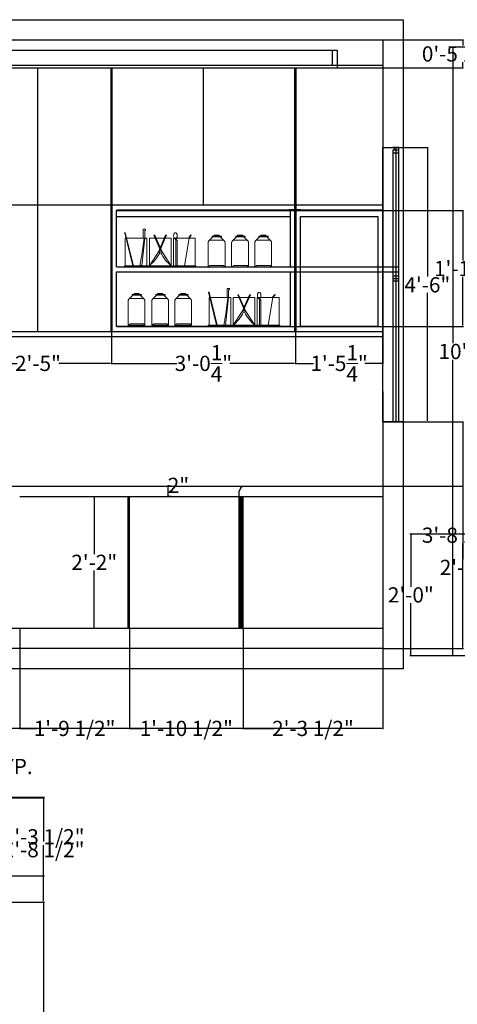
# Model space of a CAD drawing. Units: inches. Extents: x 1686244 to 1686928, y 1936095 to 1936489.
# Tile 9 of 11: x 1686616 to 1686702, y 1936281 to 1936475. Entities that reach past the tile are written whole.
import ezdxf

# ---------------------------------------------------------------- set-up
doc = ezdxf.new("R2010")
doc.units = ezdxf.units.IN
doc.header["$MEASUREMENT"] = 0
for name, color, linetype, lineweight in [('A-ANNO-DIMS', 240, 'Continuous', 18), ('A-ELEV', 7, 'Continuous', 25), ('A-FURN', 40, 'Continuous', 18)]:
    doc.layers.add(name, color=color, linetype=linetype, lineweight=lineweight)
doc.styles.get("Standard").update_dxf_attribs({"font": 'arial.ttf'})
doc.dimstyles.get("Standard").update_dxf_attribs({"dimtxt": 3, "dimasz": 0.18, "dimexe": 0.18, "dimexo": 0.0625, "dimgap": 0.09, "dimtad": 0, "dimtih": 1, "dimtoh": 1, "dimzin": 0, "dimdsep": 46, "dimlunit": 4, "dimtxsty": 'Standard', "dimcen": 0.09, "dimadec": 0, "dimazin": 0, "dimtfac": 1, "dimtofl": 0, "dimtmove": 0, "dimatfit": 3, "dimfxl": 1, "dimtolj": 1, "dimtzin": 0, "dimarcsym": 0})

# ---------------------------------------------------------------- blocks, each defined once
blk = doc.blocks.new('*D16')
at = {"layer": 'A-ANNO-DIMS', "color": 0, "lineweight": -2, "transparency": 16777216}
for p, q in [((1686604.76, 1936413.3), (1686604.76, 1936406.91)), ((1686633.76, 1936413.3), (1686633.76, 1936406.91)), ((1686604.94, 1936407.09), (1686615.16, 1936407.09)), ((1686633.58, 1936407.09), (1686623.36, 1936407.09))]:
    blk.add_line(p, q, dxfattribs=at)
at = {"layer": 'A-ANNO-DIMS', "color": 0, "transparency": 16777216}
for points in [[(1686604.94, 1936407.12), (1686604.94, 1936407.06), (1686604.76, 1936407.09)], [(1686633.58, 1936407.12), (1686633.58, 1936407.06), (1686633.76, 1936407.09)]]:
    blk.add_solid(points, dxfattribs=at)
at = {"layer": 'Defpoints', "color": 0, "transparency": 16777216}
for p in [(1686604.76, 1936413.36), (1686633.76, 1936413.36), (1686633.76, 1936407.09)]:
    blk.add_point(p, dxfattribs=at)
at = {"layer": 'A-ANNO-DIMS', "color": 0, "transparency": 16777216, "insert": (1686619.26, 1936407.09), "char_height": 3, "attachment_point": 5}
blk.add_mtext('\\A1;2\'-5"', dxfattribs=at)
blk = doc.blocks.new('*D17')
at = {"layer": 'A-ANNO-DIMS', "color": 0, "lineweight": -2, "transparency": 16777216}
for p, q in [((1686633.76, 1936413.3), (1686633.76, 1936406.91)), ((1686670.01, 1936413.3), (1686670.01, 1936406.91)), ((1686633.94, 1936407.09), (1686646.67, 1936407.09)), ((1686669.83, 1936407.09), (1686657.1, 1936407.09))]:
    blk.add_line(p, q, dxfattribs=at)
at = {"layer": 'A-ANNO-DIMS', "color": 0, "transparency": 16777216}
for points in [[(1686633.94, 1936407.12), (1686633.94, 1936407.06), (1686633.76, 1936407.09)], [(1686669.83, 1936407.12), (1686669.83, 1936407.06), (1686670.01, 1936407.09)]]:
    blk.add_solid(points, dxfattribs=at)
at = {"layer": 'Defpoints', "color": 0, "transparency": 16777216}
for p in [(1686633.76, 1936413.36), (1686670.01, 1936413.36), (1686670.01, 1936407.09)]:
    blk.add_point(p, dxfattribs=at)
at = {"layer": 'A-ANNO-DIMS', "color": 0, "transparency": 16777216, "insert": (1686651.88, 1936407.09), "char_height": 3, "attachment_point": 5}
blk.add_mtext('\\A1;3\'-0{\\H1x;\\S1/4;}"', dxfattribs=at)
blk = doc.blocks.new('*D18')
at = {"layer": 'A-ANNO-DIMS', "color": 0, "lineweight": -2, "transparency": 16777216}
for p, q in [((1686670.01, 1936413.3), (1686670.01, 1936406.91)), ((1686687.26, 1936413.3), (1686687.26, 1936406.91)), ((1686670.19, 1936407.09), (1686673.56, 1936407.09)), ((1686687.08, 1936407.09), (1686683.71, 1936407.09))]:
    blk.add_line(p, q, dxfattribs=at)
at = {"layer": 'A-ANNO-DIMS', "color": 0, "transparency": 16777216}
for points in [[(1686670.19, 1936407.12), (1686670.19, 1936407.06), (1686670.01, 1936407.09)], [(1686687.08, 1936407.12), (1686687.08, 1936407.06), (1686687.26, 1936407.09)]]:
    blk.add_solid(points, dxfattribs=at)
at = {"layer": 'Defpoints', "color": 0, "transparency": 16777216}
for p in [(1686670.01, 1936413.36), (1686687.26, 1936413.36), (1686687.26, 1936407.09)]:
    blk.add_point(p, dxfattribs=at)
at = {"layer": 'A-ANNO-DIMS', "color": 0, "transparency": 16777216, "insert": (1686678.63, 1936407.09), "char_height": 3, "attachment_point": 5}
blk.add_mtext('\\A1;1\'-5{\\H1x;\\S1/4;}"', dxfattribs=at)
blk = doc.blocks.new('*D19')
at = {"layer": 'A-ANNO-DIMS', "color": 0, "lineweight": -2, "transparency": 16777216}
for p, q in [((1686691.32, 1936449.63), (1686696.22, 1936449.63)), ((1686696.04, 1936449.45), (1686696.04, 1936424.21)), ((1686696.04, 1936395.73), (1686696.04, 1936420.97)), ((1686691.32, 1936395.55), (1686696.22, 1936395.55))]:
    blk.add_line(p, q, dxfattribs=at)
at = {"layer": 'A-ANNO-DIMS', "color": 0, "transparency": 16777216}
for points in [[(1686696.01, 1936449.45), (1686696.07, 1936449.45), (1686696.04, 1936449.63)], [(1686696.01, 1936395.73), (1686696.07, 1936395.73), (1686696.04, 1936395.55)]]:
    blk.add_solid(points, dxfattribs=at)
at = {"layer": 'Defpoints', "color": 0, "transparency": 16777216}
for p in [(1686691.26, 1936449.63), (1686691.26, 1936395.55), (1686696.04, 1936395.55)]:
    blk.add_point(p, dxfattribs=at)
at = {"layer": 'A-ANNO-DIMS', "color": 0, "transparency": 16777216, "insert": (1686696.04, 1936422.59), "char_height": 3, "attachment_point": 5}
blk.add_mtext('\\A1;4\'-6"', dxfattribs=at)
blk = doc.blocks.new('*D36')
at = {"layer": 'A-ANNO-DIMS', "color": 0, "lineweight": -2, "transparency": 16777216}
for p, q in [((1686707.26, 1936469.44), (1686700.9, 1936469.44)), ((1686701.08, 1936469.26), (1686701.08, 1936411.06)), ((1686701.08, 1936349.62), (1686701.08, 1936407.82)), ((1686707.26, 1936349.44), (1686700.9, 1936349.44))]:
    blk.add_line(p, q, dxfattribs=at)
at = {"layer": 'A-ANNO-DIMS', "color": 0, "transparency": 16777216}
for points in [[(1686701.05, 1936469.26), (1686701.11, 1936469.26), (1686701.08, 1936469.44)], [(1686701.05, 1936349.62), (1686701.11, 1936349.62), (1686701.08, 1936349.44)]]:
    blk.add_solid(points, dxfattribs=at)
at = {"layer": 'Defpoints', "color": 0, "transparency": 16777216}
for p in [(1686707.33, 1936469.44), (1686701.08, 1936349.44), (1686707.33, 1936349.44)]:
    blk.add_point(p, dxfattribs=at)
at = {"layer": 'A-ANNO-DIMS', "color": 0, "transparency": 16777216, "insert": (1686701.08, 1936409.44), "char_height": 3, "attachment_point": 5}
blk.add_mtext("\\A1;10'", dxfattribs=at)
blk = doc.blocks.new('*D61')
at = {"layer": 'A-ANNO-DIMS', "color": 0, "lineweight": -2, "transparency": 16777216}
for p, q in [((1686630.41, 1936380.86), (1686630.53, 1936380.86)), ((1686630.35, 1936380.68), (1686630.35, 1936369.46)), ((1686630.35, 1936355.04), (1686630.35, 1936366.27)), ((1686630.41, 1936354.86), (1686630.53, 1936354.86))]:
    blk.add_line(p, q, dxfattribs=at)
at = {"layer": 'A-ANNO-DIMS', "color": 0, "transparency": 16777216}
for points in [[(1686630.32, 1936380.68), (1686630.38, 1936380.68), (1686630.35, 1936380.86)], [(1686630.32, 1936355.04), (1686630.38, 1936355.04), (1686630.35, 1936354.86)]]:
    blk.add_solid(points, dxfattribs=at)
at = {"layer": 'Defpoints', "color": 0, "transparency": 16777216}
for p in [(1686630.35, 1936380.86), (1686630.35, 1936380.86), (1686630.35, 1936354.86)]:
    blk.add_point(p, dxfattribs=at)
at = {"layer": 'A-ANNO-DIMS', "color": 0, "transparency": 16777216, "insert": (1686630.35, 1936367.86), "char_height": 3, "attachment_point": 5}
blk.add_mtext('\\A1;2\'-2"', dxfattribs=at)
blk = doc.blocks.new('*D62')
at = {"layer": 'A-ANNO-DIMS', "color": 0, "lineweight": -2, "transparency": 16777216}
for p, q in [((1686645.52, 1936382.86), (1686644.76, 1936382.86)), ((1686644.94, 1936382.86), (1686644.94, 1936383.04)), ((1686644.94, 1936383.04), (1686645.12, 1936383.04)), ((1686645.52, 1936380.86), (1686644.76, 1936380.86)), ((1686644.94, 1936381.04), (1686644.94, 1936382.68))]:
    blk.add_line(p, q, dxfattribs=at)
at = {"layer": 'A-ANNO-DIMS', "color": 0, "transparency": 16777216}
for points in [[(1686644.91, 1936382.68), (1686644.97, 1936382.68), (1686644.94, 1936382.86)], [(1686644.91, 1936381.04), (1686644.97, 1936381.04), (1686644.94, 1936380.86)]]:
    blk.add_solid(points, dxfattribs=at)
at = {"layer": 'Defpoints', "color": 0, "transparency": 16777216}
for p in [(1686644.94, 1936382.86), (1686645.58, 1936382.86), (1686645.58, 1936380.86)]:
    blk.add_point(p, dxfattribs=at)
at = {"layer": 'A-ANNO-DIMS', "color": 0, "transparency": 16777216, "insert": (1686646.96, 1936383.04), "char_height": 3, "attachment_point": 5}
blk.add_mtext('\\A1;2"', dxfattribs=at)
blk = doc.blocks.new('*D67')
at = {"layer": 'A-ANNO-DIMS', "color": 0, "lineweight": -2, "transparency": 16777216}
for p, q in [((1686559.57, 1936329.98), (1686559.57, 1936327.43)), ((1686575.74, 1936329.98), (1686575.74, 1936327.43)), ((1686559.75, 1936327.61), (1686575.56, 1936327.61)), ((1686575.74, 1936327.61), (1686575.92, 1936327.61))]:
    blk.add_line(p, q, dxfattribs=at)
at = {"layer": 'A-ANNO-DIMS', "color": 0, "transparency": 16777216}
for points in [[(1686559.75, 1936327.64), (1686559.75, 1936327.58), (1686559.57, 1936327.61)], [(1686575.56, 1936327.64), (1686575.56, 1936327.58), (1686575.74, 1936327.61)]]:
    blk.add_solid(points, dxfattribs=at)
at = {"layer": 'Defpoints', "color": 0, "transparency": 16777216}
for p in [(1686559.57, 1936330.04), (1686575.74, 1936330.04), (1686575.74, 1936327.61)]:
    blk.add_point(p, dxfattribs=at)
at = {"layer": 'A-ANNO-DIMS', "color": 0, "transparency": 16777216, "insert": (1686597.66, 1936327.61), "char_height": 3, "attachment_point": 5}
blk.add_mtext('\\A1;BAR STOOL 1\'-4" TYP.', dxfattribs=at)
blk = doc.blocks.new('*D97')
at = {"layer": 'A-ANNO-DIMS', "color": 0, "lineweight": -2, "transparency": 16777216}
for p, q in [((1686481.26, 1936350.8), (1686481.26, 1936334.93)), ((1686687.26, 1936350.8), (1686687.26, 1936334.93)), ((1686481.44, 1936335.11), (1686579.16, 1936335.11)), ((1686687.08, 1936335.11), (1686589.36, 1936335.11))]:
    blk.add_line(p, q, dxfattribs=at)
at = {"layer": 'A-ANNO-DIMS', "color": 0, "transparency": 16777216}
for points in [[(1686481.44, 1936335.14), (1686481.44, 1936335.08), (1686481.26, 1936335.11)], [(1686687.08, 1936335.14), (1686687.08, 1936335.08), (1686687.26, 1936335.11)]]:
    blk.add_solid(points, dxfattribs=at)
at = {"layer": 'Defpoints', "color": 0, "transparency": 16777216}
for p in [(1686481.26, 1936350.86), (1686687.26, 1936350.86), (1686687.26, 1936335.11)]:
    blk.add_point(p, dxfattribs=at)
at = {"layer": 'A-ANNO-DIMS', "color": 0, "transparency": 16777216, "insert": (1686584.26, 1936335.11), "char_height": 3, "attachment_point": 5}
blk.add_mtext('\\A1;17\'-2"', dxfattribs=at)
blk = doc.blocks.new('*D99')
at = {"layer": 'A-ANNO-DIMS', "color": 0, "lineweight": -2, "transparency": 16777216}
for p, q in [((1686615.66, 1936354.8), (1686615.66, 1936334.93)), ((1686637.31, 1936354.8), (1686637.31, 1936334.93)), ((1686615.84, 1936335.11), (1686619.05, 1936335.11)), ((1686637.13, 1936335.11), (1686633.91, 1936335.11))]:
    blk.add_line(p, q, dxfattribs=at)
at = {"layer": 'A-ANNO-DIMS', "color": 0, "transparency": 16777216}
for points in [[(1686615.84, 1936335.14), (1686615.84, 1936335.08), (1686615.66, 1936335.11)], [(1686637.13, 1936335.14), (1686637.13, 1936335.08), (1686637.31, 1936335.11)]]:
    blk.add_solid(points, dxfattribs=at)
at = {"layer": 'Defpoints', "color": 0, "transparency": 16777216}
for p in [(1686615.66, 1936354.86), (1686637.31, 1936354.86), (1686637.31, 1936335.11)]:
    blk.add_point(p, dxfattribs=at)
at = {"layer": 'A-ANNO-DIMS', "color": 0, "transparency": 16777216, "insert": (1686626.48, 1936335.11), "char_height": 3, "attachment_point": 5}
blk.add_mtext('\\A1;1\'-9 1/2"', dxfattribs=at)
blk = doc.blocks.new('*D100')
at = {"layer": 'A-ANNO-DIMS', "color": 0, "lineweight": -2, "transparency": 16777216}
for p, q in [((1686637.31, 1936354.8), (1686637.31, 1936334.93)), ((1686659.71, 1936354.8), (1686659.71, 1936334.93)), ((1686637.49, 1936335.11), (1686639.91, 1936335.11)), ((1686659.53, 1936335.11), (1686657.11, 1936335.11))]:
    blk.add_line(p, q, dxfattribs=at)
at = {"layer": 'A-ANNO-DIMS', "color": 0, "transparency": 16777216}
for points in [[(1686637.49, 1936335.14), (1686637.49, 1936335.08), (1686637.31, 1936335.11)], [(1686659.53, 1936335.14), (1686659.53, 1936335.08), (1686659.71, 1936335.11)]]:
    blk.add_solid(points, dxfattribs=at)
at = {"layer": 'Defpoints', "color": 0, "transparency": 16777216}
for p in [(1686637.31, 1936354.86), (1686659.71, 1936354.86), (1686659.71, 1936335.11)]:
    blk.add_point(p, dxfattribs=at)
at = {"layer": 'A-ANNO-DIMS', "color": 0, "transparency": 16777216, "insert": (1686648.51, 1936335.11), "char_height": 3, "attachment_point": 5}
blk.add_mtext('\\A1;1\'-10 1/2"', dxfattribs=at)
blk = doc.blocks.new('*D101')
at = {"layer": 'A-ANNO-DIMS', "color": 0, "lineweight": -2, "transparency": 16777216}
for p, q in [((1686659.71, 1936354.8), (1686659.71, 1936334.93)), ((1686687.26, 1936354.8), (1686687.26, 1936334.93)), ((1686659.89, 1936335.11), (1686665.89, 1936335.11)), ((1686687.08, 1936335.11), (1686681.08, 1936335.11))]:
    blk.add_line(p, q, dxfattribs=at)
at = {"layer": 'A-ANNO-DIMS', "color": 0, "transparency": 16777216}
for points in [[(1686659.89, 1936335.14), (1686659.89, 1936335.08), (1686659.71, 1936335.11)], [(1686687.08, 1936335.14), (1686687.08, 1936335.08), (1686687.26, 1936335.11)]]:
    blk.add_solid(points, dxfattribs=at)
at = {"layer": 'Defpoints', "color": 0, "transparency": 16777216}
for p in [(1686659.71, 1936354.86), (1686687.26, 1936354.86), (1686687.26, 1936335.11)]:
    blk.add_point(p, dxfattribs=at)
at = {"layer": 'A-ANNO-DIMS', "color": 0, "transparency": 16777216, "insert": (1686673.48, 1936335.11), "char_height": 3, "attachment_point": 5}
blk.add_mtext('\\A1;2\'-3 1/2"', dxfattribs=at)
blk = doc.blocks.new('*D102')
at = {"layer": 'A-ANNO-DIMS', "color": 0, "lineweight": -2, "transparency": 16777216}
for p, q in [((1686687.32, 1936395.55), (1686703.19, 1936395.55)), ((1686703.01, 1936395.37), (1686703.01, 1936374.85)), ((1686703.01, 1936351.04), (1686703.01, 1936371.57)), ((1686687.32, 1936350.86), (1686703.19, 1936350.86))]:
    blk.add_line(p, q, dxfattribs=at)
at = {"layer": 'A-ANNO-DIMS', "color": 0, "transparency": 16777216}
for points in [[(1686702.98, 1936395.37), (1686703.04, 1936395.37), (1686703.01, 1936395.55)], [(1686702.98, 1936351.04), (1686703.04, 1936351.04), (1686703.01, 1936350.86)]]:
    blk.add_solid(points, dxfattribs=at)
at = {"layer": 'Defpoints', "color": 0, "transparency": 16777216}
for p in [(1686687.26, 1936395.55), (1686687.26, 1936350.86), (1686703.01, 1936350.86)]:
    blk.add_point(p, dxfattribs=at)
at = {"layer": 'A-ANNO-DIMS', "color": 0, "transparency": 16777216, "insert": (1686703.01, 1936373.21), "char_height": 3, "attachment_point": 5}
blk.add_mtext('\\A1;3\'-8 1/2"', dxfattribs=at)
blk = doc.blocks.new('*D103')
at = {"layer": 'A-ANNO-DIMS', "color": 0, "lineweight": -2, "transparency": 16777216}
for p, q in [((1686687.32, 1936382.86), (1686703.19, 1936382.86)), ((1686703.01, 1936382.68), (1686703.01, 1936368.49)), ((1686703.01, 1936351.04), (1686703.01, 1936365.24)), ((1686687.32, 1936350.86), (1686703.19, 1936350.86))]:
    blk.add_line(p, q, dxfattribs=at)
at = {"layer": 'A-ANNO-DIMS', "color": 0, "transparency": 16777216}
for points in [[(1686702.98, 1936382.68), (1686703.04, 1936382.68), (1686703.01, 1936382.86)], [(1686702.98, 1936351.04), (1686703.04, 1936351.04), (1686703.01, 1936350.86)]]:
    blk.add_solid(points, dxfattribs=at)
at = {"layer": 'Defpoints', "color": 0, "transparency": 16777216}
for p in [(1686687.26, 1936382.86), (1686687.26, 1936350.86), (1686703.01, 1936350.86)]:
    blk.add_point(p, dxfattribs=at)
at = {"layer": 'A-ANNO-DIMS', "color": 0, "transparency": 16777216, "insert": (1686703.01, 1936366.86), "char_height": 3, "attachment_point": 5}
blk.add_mtext('\\A1;2\'-8"', dxfattribs=at)
blk = doc.blocks.new('*D104')
at = {"layer": 'A-ANNO-DIMS', "color": 0, "lineweight": -2, "transparency": 16777216}
for p, q in [((1686687.32, 1936470.86), (1686703.19, 1936470.86)), ((1686703.01, 1936470.68), (1686703.01, 1936469.75)), ((1686703.01, 1936465.54), (1686703.01, 1936466.47)), ((1686687.32, 1936465.36), (1686703.19, 1936465.36))]:
    blk.add_line(p, q, dxfattribs=at)
at = {"layer": 'A-ANNO-DIMS', "color": 0, "transparency": 16777216}
for points in [[(1686702.98, 1936470.68), (1686703.04, 1936470.68), (1686703.01, 1936470.86)], [(1686702.98, 1936465.54), (1686703.04, 1936465.54), (1686703.01, 1936465.36)]]:
    blk.add_solid(points, dxfattribs=at)
at = {"layer": 'Defpoints', "color": 0, "transparency": 16777216}
for p in [(1686687.26, 1936470.86), (1686687.26, 1936465.36), (1686703.01, 1936465.36)]:
    blk.add_point(p, dxfattribs=at)
at = {"layer": 'A-ANNO-DIMS', "color": 0, "transparency": 16777216, "insert": (1686703.01, 1936468.11), "char_height": 3, "attachment_point": 5}
blk.add_mtext('\\A1;0\'-5 1/2"', dxfattribs=at)
blk = doc.blocks.new('*D105')
at = {"layer": 'A-ANNO-DIMS', "color": 0, "lineweight": -2, "transparency": 16777216}
for p, q in [((1686634.84, 1936437.21), (1686703.19, 1936437.21)), ((1686703.01, 1936437.03), (1686703.01, 1936427.38)), ((1686703.01, 1936414.54), (1686703.01, 1936424.19)), ((1686634.82, 1936414.36), (1686703.19, 1936414.36))]:
    blk.add_line(p, q, dxfattribs=at)
at = {"layer": 'A-ANNO-DIMS', "color": 0, "transparency": 16777216}
for points in [[(1686702.98, 1936437.03), (1686703.04, 1936437.03), (1686703.01, 1936437.21)], [(1686702.98, 1936414.54), (1686703.04, 1936414.54), (1686703.01, 1936414.36)]]:
    blk.add_solid(points, dxfattribs=at)
at = {"layer": 'Defpoints', "color": 0, "transparency": 16777216}
for p in [(1686634.78, 1936437.21), (1686634.76, 1936414.36), (1686703.01, 1936414.36)]:
    blk.add_point(p, dxfattribs=at)
at = {"layer": 'A-ANNO-DIMS', "color": 0, "transparency": 16777216, "insert": (1686703.01, 1936425.79), "char_height": 3, "attachment_point": 5}
blk.add_mtext('\\A1;1\'-11"', dxfattribs=at)
blk = doc.blocks.new('*D111')
at = {"layer": 'A-ANNO-DIMS', "color": 0, "lineweight": -2, "transparency": 16777216}
for p, q in [((1686707.26, 1936373.44), (1686692.6, 1936373.44)), ((1686692.78, 1936373.26), (1686692.78, 1936363.06)), ((1686692.78, 1936349.62), (1686692.78, 1936359.82)), ((1686707.26, 1936349.44), (1686692.6, 1936349.44))]:
    blk.add_line(p, q, dxfattribs=at)
at = {"layer": 'A-ANNO-DIMS', "color": 0, "transparency": 16777216}
for points in [[(1686692.75, 1936373.26), (1686692.81, 1936373.26), (1686692.78, 1936373.44)], [(1686692.75, 1936349.62), (1686692.81, 1936349.62), (1686692.78, 1936349.44)]]:
    blk.add_solid(points, dxfattribs=at)
at = {"layer": 'Defpoints', "color": 0, "transparency": 16777216}
for p in [(1686692.78, 1936373.44), (1686707.33, 1936373.44), (1686707.33, 1936349.44)]:
    blk.add_point(p, dxfattribs=at)
at = {"layer": 'A-ANNO-DIMS', "color": 0, "transparency": 16777216, "insert": (1686692.78, 1936361.44), "char_height": 3, "attachment_point": 5}
blk.add_mtext('\\A1;2\'-0"', dxfattribs=at)
blk = doc.blocks.new('*D120')
at = {"layer": 'A-ANNO-DIMS', "color": 0, "lineweight": -2, "transparency": 16777216}
for p, q in [((1686599.41, 1936300.86), (1686620.56, 1936300.86)), ((1686620.38, 1936300.68), (1686620.38, 1936215.99)), ((1686620.38, 1936128.04), (1686620.38, 1936212.74)), ((1686599.41, 1936127.86), (1686620.56, 1936127.86))]:
    blk.add_line(p, q, dxfattribs=at)
at = {"layer": 'A-ANNO-DIMS', "color": 0, "transparency": 16777216}
for points in [[(1686620.35, 1936300.68), (1686620.41, 1936300.68), (1686620.38, 1936300.86)], [(1686620.35, 1936128.04), (1686620.41, 1936128.04), (1686620.38, 1936127.86)]]:
    blk.add_solid(points, dxfattribs=at)
at = {"layer": 'Defpoints', "color": 0, "transparency": 16777216}
for p in [(1686599.35, 1936300.86), (1686599.35, 1936127.86), (1686620.38, 1936127.86)]:
    blk.add_point(p, dxfattribs=at)
at = {"layer": 'A-ANNO-DIMS', "color": 0, "transparency": 16777216, "insert": (1686620.38, 1936214.36), "char_height": 3, "attachment_point": 5}
blk.add_mtext('\\A1;14\'-5"', dxfattribs=at)
blk = doc.blocks.new('*D125')
at = {"layer": 'A-ANNO-DIMS', "color": 0, "lineweight": -2, "transparency": 16777216}
for p, q in [((1686563.48, 1936321.54), (1686620.56, 1936321.54)), ((1686620.38, 1936321.36), (1686620.38, 1936312.84)), ((1686620.38, 1936301.04), (1686620.38, 1936309.56)), ((1686563.48, 1936300.86), (1686620.56, 1936300.86))]:
    blk.add_line(p, q, dxfattribs=at)
at = {"layer": 'A-ANNO-DIMS', "color": 0, "transparency": 16777216}
for points in [[(1686620.35, 1936321.36), (1686620.41, 1936321.36), (1686620.38, 1936321.54)], [(1686620.35, 1936301.04), (1686620.41, 1936301.04), (1686620.38, 1936300.86)]]:
    blk.add_solid(points, dxfattribs=at)
at = {"layer": 'Defpoints', "color": 0, "transparency": 16777216}
for p in [(1686563.41, 1936321.54), (1686563.41, 1936300.86), (1686620.38, 1936300.86)]:
    blk.add_point(p, dxfattribs=at)
at = {"layer": 'A-ANNO-DIMS', "color": 0, "transparency": 16777216, "insert": (1686620.38, 1936311.2), "char_height": 3, "attachment_point": 5}
blk.add_mtext('\\A1;1\'-8 1/2"', dxfattribs=at)
blk = doc.blocks.new('*D126')
at = {"layer": 'A-ANNO-DIMS', "color": 0, "lineweight": -2, "transparency": 16777216}
for p, q in [((1686608.41, 1936321.45), (1686620.56, 1936321.45)), ((1686620.38, 1936321.27), (1686620.38, 1936315.38)), ((1686620.38, 1936306.21), (1686620.38, 1936312.1)), ((1686608.39, 1936306.03), (1686620.56, 1936306.03))]:
    blk.add_line(p, q, dxfattribs=at)
at = {"layer": 'A-ANNO-DIMS', "color": 0, "transparency": 16777216}
for points in [[(1686620.35, 1936321.27), (1686620.41, 1936321.27), (1686620.38, 1936321.45)], [(1686620.35, 1936306.21), (1686620.41, 1936306.21), (1686620.38, 1936306.03)]]:
    blk.add_solid(points, dxfattribs=at)
at = {"layer": 'Defpoints', "color": 0, "transparency": 16777216}
for p in [(1686608.35, 1936321.45), (1686608.32, 1936306.03), (1686620.38, 1936306.03)]:
    blk.add_point(p, dxfattribs=at)
at = {"layer": 'A-ANNO-DIMS', "color": 0, "transparency": 16777216, "insert": (1686620.38, 1936313.74), "char_height": 3, "attachment_point": 5}
blk.add_mtext('\\A1;1\'-3 1/2"', dxfattribs=at)

msp = doc.modelspace()

# ---------------------------------------------------------------- linework, layer by layer
at = {"layer": 'A-ELEV'}
for p, q in [((1686509.758, 1936468.864), (1686678.258, 1936468.864)), ((1686677.258, 1936468.864), (1686677.258, 1936465.864)), ((1686481.258, 1936465.864), (1686687.259, 1936465.864)), ((1686481.258, 1936465.364), (1686687.259, 1936465.364)), ((1686619.258, 1936413.364), (1686619.258, 1936465.364)), ((1686651.883, 1936438.364), (1686651.883, 1936465.364)), ((1686690.42, 1936449.122), (1686689.259, 1936449.122)), ((1686689.527, 1936449.122), (1686689.527, 1936449.629)), ((1686689.84, 1936449.629), (1686689.84, 1936395.551)), ((1686690.42, 1936448.574), (1686689.259, 1936448.574)), ((1686509.758, 1936438.364), (1686687.259, 1936438.364)), ((1686671.008, 1936437.364), (1686668.758, 1936437.364)), ((1686686.259, 1936437.364), (1686687.259, 1936437.364)), ((1686634.758, 1936436.051), (1686669.008, 1936436.051)), ((1686671.008, 1936436.051), (1686686.259, 1936436.051)), ((1686634.758, 1936426.114), (1686671.008, 1936426.114)), ((1686671.008, 1936426.114), (1686690.42, 1936426.114)), ((1686634.758, 1936425.114), (1686671.008, 1936425.114)), ((1686671.008, 1936425.114), (1686690.42, 1936425.114)), ((1686689.259, 1936424.338), (1686690.42, 1936424.338)), ((1686689.259, 1936423.838), (1686690.42, 1936423.838)), ((1686689.259, 1936423.338), (1686690.42, 1936423.338)), ((1686509.758, 1936413.364), (1686687.259, 1936413.364)), ((1686509.758, 1936412.364), (1686687.259, 1936412.364)), ((1686687.259, 1936401.547), (1686687.259, 1936346.864)), ((1686509.758, 1936382.864), (1686687.259, 1936382.864)), ((1686659.958, 1936382.864), (1686687.259, 1936382.864)), ((1686615.658, 1936380.864), (1686687.259, 1936380.864)), ((1686637.058, 1936354.864), (1686637.058, 1936380.864)), ((1686637.308, 1936354.864), (1686637.308, 1936380.864)), ((1686658.958, 1936380.864), (1686658.958, 1936381.864)), ((1686658.958, 1936354.864), (1686658.958, 1936380.864)), ((1686659.208, 1936354.864), (1686659.208, 1936380.864)), ((1686659.458, 1936354.864), (1686659.458, 1936380.864)), ((1686659.708, 1936354.864), (1686659.708, 1936380.864)), ((1686658.958, 1936375.367), (1686659.708, 1936375.367)), ((1686658.958, 1936369.403), (1686659.708, 1936369.403)), ((1686509.758, 1936354.864), (1686687.259, 1936354.864)), ((1686659.708, 1936354.864), (1686659.708, 1936350.864))]:
    msp.add_line(p, q, dxfattribs=at)
for points in [[(1686691.259, 1936346.864), (1686476.258, 1936346.864), (1686476.258, 1936474.864), (1686691.259, 1936474.864)], [(1686687.259, 1936449.629), (1686691.259, 1936449.629), (1686691.259, 1936395.551), (1686687.259, 1936395.552)]]:
    msp.add_lwpolyline(points, close=True, dxfattribs=at)
for points in [[(1686687.259, 1936354.864), (1686687.259, 1936350.864), (1686480.258, 1936350.864), (1686480.258, 1936470.864), (1686687.259, 1936470.864), (1686687.259, 1936412.364)], [(1686678.258, 1936468.864), (1686678.258, 1936465.364)], [(1686689.259, 1936449.122), (1686689.259, 1936395.551), (1686690.42, 1936395.551), (1686690.42, 1936449.629), (1686689.259, 1936449.629)], [(1686671.008, 1936437.364), (1686686.259, 1936437.364)], [(1686686.259, 1936436.051), (1686686.259, 1936414.364), (1686671.008, 1936414.364), (1686671.008, 1936436.051)], [(1686669.008, 1936425.114), (1686669.008, 1936414.364), (1686634.758, 1936414.364), (1686634.758, 1936425.114)]]:
    msp.add_lwpolyline(points, dxfattribs=at)
at = {"layer": 'A-ELEV', "const_width": 0.5}
for points in [[(1686633.758, 1936413.364), (1686633.758, 1936465.364)], [(1686670.008, 1936413.364), (1686670.008, 1936465.364)]]:
    msp.add_lwpolyline(points, dxfattribs=at)
at = {"layer": 'A-ELEV'}
msp.add_lwpolyline([(1686634.758, 1936426.114), (1686634.758, 1936437.114, -0.4142136), (1686635.008, 1936437.364), (1686668.758, 1936437.364, -0.4142136), (1686669.008, 1936437.114), (1686669.008, 1936426.114)], format="xyb", dxfattribs=at)
msp.add_arc((1686659.958, 1936381.864), 1, 90, 180, dxfattribs=at)
at = {"layer": 'A-FURN'}
for p, q in [((1686636.358, 1936432.862), (1686636.477, 1936432.875)), ((1686637.941, 1936426.355), (1686636.358, 1936432.862)), ((1686636.477, 1936432.875), (1686638.076, 1936426.355)), ((1686649.048, 1936431.815), (1686648.122, 1936426.355)), ((1686648.122, 1936426.355), (1686649.048, 1936431.815)), ((1686649.011, 1936431.851), (1686649.41, 1936432.437)), ((1686649.048, 1936431.815), (1686649.011, 1936431.851)), ((1686649.072, 1936431.791), (1686649.048, 1936431.815)), ((1686649.475, 1936432.372), (1686649.072, 1936431.791)), ((1686649.41, 1936432.437), (1686649.475, 1936432.372)), ((1686652.951, 1936431.242), (1686653.764, 1936432.056)), ((1686653.885, 1936432.183), (1686654.044, 1936432.357)), ((1686654.044, 1936432.357), (1686654.936, 1936432.357)), ((1686654.936, 1936432.357), (1686655.084, 1936432.183)), ((1686655.992, 1936431.242), (1686655.212, 1936432.057)), ((1686657.6, 1936431.242), (1686658.413, 1936432.056)), ((1686658.533, 1936432.183), (1686658.693, 1936432.357)), ((1686658.693, 1936432.357), (1686659.585, 1936432.357)), ((1686659.585, 1936432.357), (1686659.733, 1936432.183)), ((1686660.641, 1936431.242), (1686659.861, 1936432.057)), ((1686662.147, 1936431.242), (1686662.96, 1936432.056)), ((1686663.081, 1936432.183), (1686663.24, 1936432.357)), ((1686663.24, 1936432.357), (1686664.132, 1936432.357)), ((1686664.132, 1936432.357), (1686664.28, 1936432.183)), ((1686665.188, 1936431.242), (1686664.408, 1936432.057)), ((1686643.011, 1936429.089), (1686641.22, 1936426.355)), ((1686643.724, 1936429.089), (1686645.515, 1936426.355)), ((1686636.463, 1936426.355), (1686636.313, 1936426.355)), ((1686636.313, 1936426.355), (1686636.313, 1936426.205)), ((1686636.313, 1936426.205), (1686640.757, 1936426.205)), ((1686640.907, 1936426.355), (1686640.757, 1936426.355)), ((1686640.757, 1936426.205), (1686640.907, 1936426.205)), ((1686640.907, 1936426.205), (1686640.907, 1936426.355)), ((1686641.22, 1936426.355), (1686641.07, 1936426.355)), ((1686641.07, 1936426.355), (1686641.07, 1936426.205)), ((1686641.07, 1936426.205), (1686645.515, 1936426.205)), ((1686645.665, 1936426.355), (1686645.515, 1936426.355)), ((1686645.515, 1936426.205), (1686645.665, 1936426.205)), ((1686645.665, 1936426.205), (1686645.665, 1936426.355)), ((1686645.975, 1936426.355), (1686645.825, 1936426.355)), ((1686645.825, 1936426.355), (1686645.825, 1936426.205)), ((1686645.825, 1936426.205), (1686650.27, 1936426.205)), ((1686650.42, 1936426.355), (1686650.27, 1936426.355)), ((1686650.27, 1936426.205), (1686650.42, 1936426.205)), ((1686650.42, 1936426.205), (1686650.42, 1936426.355)), ((1686652.805, 1936426.114), (1686653.208, 1936426.362)), ((1686653.208, 1936426.362), (1686655.84, 1936426.362)), ((1686655.84, 1936426.362), (1686656.139, 1936426.114)), ((1686657.453, 1936426.114), (1686657.856, 1936426.362)), ((1686657.856, 1936426.362), (1686660.489, 1936426.362)), ((1686660.489, 1936426.362), (1686660.787, 1936426.114)), ((1686662.001, 1936426.114), (1686662.404, 1936426.362)), ((1686662.404, 1936426.362), (1686665.036, 1936426.362)), ((1686665.036, 1936426.362), (1686665.335, 1936426.114)), ((1686637.178, 1936419.739), (1686637.991, 1936420.552)), ((1686638.111, 1936420.679), (1686638.27, 1936420.854)), ((1686638.27, 1936420.854), (1686639.162, 1936420.854)), ((1686639.162, 1936420.854), (1686639.311, 1936420.679)), ((1686640.219, 1936419.739), (1686639.438, 1936420.553)), ((1686641.826, 1936419.739), (1686642.639, 1936420.552)), ((1686642.76, 1936420.679), (1686642.919, 1936420.854)), ((1686642.919, 1936420.854), (1686643.811, 1936420.854)), ((1686643.811, 1936420.854), (1686643.959, 1936420.679)), ((1686644.867, 1936419.739), (1686644.087, 1936420.553)), ((1686646.374, 1936419.739), (1686647.187, 1936420.552)), ((1686647.307, 1936420.679), (1686647.466, 1936420.854)), ((1686647.466, 1936420.854), (1686648.358, 1936420.854)), ((1686648.358, 1936420.854), (1686648.507, 1936420.679)), ((1686649.415, 1936419.739), (1686648.634, 1936420.553)), ((1686652.883, 1936421.127), (1686653.002, 1936421.14)), ((1686654.466, 1936414.62), (1686652.883, 1936421.127)), ((1686653.002, 1936421.14), (1686654.601, 1936414.62)), ((1686665.573, 1936420.079), (1686664.647, 1936414.62)), ((1686664.647, 1936414.62), (1686665.573, 1936420.079)), ((1686665.536, 1936420.116), (1686665.935, 1936420.702)), ((1686665.573, 1936420.079), (1686665.536, 1936420.116)), ((1686665.596, 1936420.056), (1686665.573, 1936420.079)), ((1686666, 1936420.637), (1686665.596, 1936420.056)), ((1686665.935, 1936420.702), (1686666, 1936420.637)), ((1686659.536, 1936417.353), (1686657.745, 1936414.62)), ((1686660.249, 1936417.353), (1686662.039, 1936414.62)), ((1686637.031, 1936414.61), (1686637.434, 1936414.858)), ((1686637.434, 1936414.858), (1686640.067, 1936414.858)), ((1686640.067, 1936414.858), (1686640.365, 1936414.61)), ((1686641.68, 1936414.61), (1686642.083, 1936414.858)), ((1686642.083, 1936414.858), (1686644.715, 1936414.858)), ((1686644.715, 1936414.858), (1686645.014, 1936414.61)), ((1686646.227, 1936414.61), (1686646.63, 1936414.858)), ((1686646.63, 1936414.858), (1686649.263, 1936414.858)), ((1686649.263, 1936414.858), (1686649.561, 1936414.61)), ((1686652.988, 1936414.62), (1686652.838, 1936414.62)), ((1686652.838, 1936414.62), (1686652.838, 1936414.47)), ((1686652.838, 1936414.47), (1686657.282, 1936414.47)), ((1686657.432, 1936414.62), (1686657.282, 1936414.62)), ((1686657.282, 1936414.47), (1686657.432, 1936414.47)), ((1686657.432, 1936414.47), (1686657.432, 1936414.62)), ((1686657.745, 1936414.62), (1686657.595, 1936414.62)), ((1686657.595, 1936414.62), (1686657.595, 1936414.47)), ((1686657.595, 1936414.47), (1686662.039, 1936414.47)), ((1686662.19, 1936414.62), (1686662.039, 1936414.62)), ((1686662.039, 1936414.47), (1686662.19, 1936414.47)), ((1686662.19, 1936414.47), (1686662.19, 1936414.62)), ((1686662.5, 1936414.62), (1686662.35, 1936414.62)), ((1686662.35, 1936414.62), (1686662.35, 1936414.47)), ((1686662.35, 1936414.47), (1686666.794, 1936414.47)), ((1686666.945, 1936414.62), (1686666.794, 1936414.62)), ((1686666.794, 1936414.47), (1686666.945, 1936414.47)), ((1686666.945, 1936414.47), (1686666.945, 1936414.62))]:
    msp.add_line(p, q, dxfattribs=at)
for points in [[(1686639.358, 1936426.355), (1686639.51, 1936427.021), (1686639.568, 1936427.272), (1686639.568, 1936427.527), (1686639.751, 1936428.527), (1686640.169, 1936431.815), (1686640.029, 1936431.815), (1686640.029, 1936433.577), (1686640.485, 1936433.577), (1686640.485, 1936433.312), (1686640.321, 1936433.312), (1686640.321, 1936431.815), (1686639.713, 1936426.355), (1686639.376, 1936426.432)], [(1686642.113, 1936432.373), (1686642.307, 1936432.373), (1686643.724, 1936429.089), (1686643.573, 1936429.004), (1686642.118, 1936432.373)], [(1686644.622, 1936432.373), (1686644.429, 1936432.373), (1686643.011, 1936429.089), (1686643.162, 1936429.004), (1686644.617, 1936432.373)], [(1686646.216, 1936431.704), (1686646.449, 1936431.299), (1686646.449, 1936426.355), (1686646.689, 1936426.355), (1686646.689, 1936431.3), (1686646.437, 1936431.657)], [(1686643.162, 1936429.004), (1686643.26, 1936428.906)], [(1686643.573, 1936429.004), (1686643.475, 1936428.906)], [(1686655.883, 1936414.62), (1686656.035, 1936415.285), (1686656.092, 1936415.537), (1686656.092, 1936415.792), (1686656.276, 1936416.791), (1686656.694, 1936420.079), (1686656.554, 1936420.079), (1686656.554, 1936421.842), (1686657.01, 1936421.842), (1686657.01, 1936421.576), (1686656.846, 1936421.576), (1686656.846, 1936420.079), (1686656.238, 1936414.62), (1686655.901, 1936414.697)], [(1686658.638, 1936420.637), (1686658.831, 1936420.637), (1686660.249, 1936417.353), (1686660.098, 1936417.269), (1686658.643, 1936420.637)], [(1686661.147, 1936420.637), (1686660.953, 1936420.637), (1686659.536, 1936417.353), (1686659.687, 1936417.269), (1686661.142, 1936420.637)], [(1686662.741, 1936419.969), (1686662.974, 1936419.564), (1686662.974, 1936414.62), (1686663.214, 1936414.62), (1686663.214, 1936419.565), (1686662.962, 1936419.922)], [(1686659.687, 1936417.269), (1686659.785, 1936417.171)], [(1686660.098, 1936417.269), (1686660, 1936417.171)]]:
    msp.add_lwpolyline(points, dxfattribs=at)
for points in [[(1686636.463, 1936431.815), (1686640.757, 1936431.815), (1686640.757, 1936426.355), (1686636.463, 1936426.355)], [(1686641.22, 1936431.815), (1686645.515, 1936431.815), (1686645.515, 1936426.355), (1686641.22, 1936426.355)], [(1686645.975, 1936431.815), (1686650.27, 1936431.815), (1686650.27, 1936426.355), (1686645.975, 1936426.355)], [(1686653.597, 1936432.183), (1686655.436, 1936432.183), (1686655.436, 1936432.057), (1686653.597, 1936432.057)], [(1686658.246, 1936432.183), (1686660.084, 1936432.183), (1686660.084, 1936432.057), (1686658.246, 1936432.057)], [(1686662.793, 1936432.183), (1686664.632, 1936432.183), (1686664.632, 1936432.057), (1686662.793, 1936432.057)], [(1686637.824, 1936420.679), (1686639.662, 1936420.679), (1686639.662, 1936420.553), (1686637.824, 1936420.553)], [(1686642.472, 1936420.679), (1686644.311, 1936420.679), (1686644.311, 1936420.553), (1686642.472, 1936420.553)], [(1686647.02, 1936420.679), (1686648.858, 1936420.679), (1686648.858, 1936420.553), (1686647.02, 1936420.553)], [(1686652.988, 1936420.079), (1686657.282, 1936420.079), (1686657.282, 1936414.62), (1686652.988, 1936414.62)], [(1686657.745, 1936420.079), (1686662.039, 1936420.079), (1686662.039, 1936414.62), (1686657.745, 1936414.62)], [(1686662.5, 1936420.079), (1686666.794, 1936420.079), (1686666.794, 1936414.62), (1686662.5, 1936414.62)]]:
    msp.add_lwpolyline(points, close=True, dxfattribs=at)
for points in [[(1686653.305, 1936431.389), (1686655.639, 1936431.389, -0.4142136), (1686656.139, 1936430.889), (1686656.139, 1936426.114), (1686652.805, 1936426.114), (1686652.805, 1936430.889, -0.4142136)], [(1686657.953, 1936431.389), (1686660.287, 1936431.389, -0.4142136), (1686660.787, 1936430.889), (1686660.787, 1936426.114), (1686657.453, 1936426.114), (1686657.453, 1936430.889, -0.4142136)], [(1686662.501, 1936431.389), (1686664.835, 1936431.389, -0.4142136), (1686665.335, 1936430.889), (1686665.335, 1936426.114), (1686662.001, 1936426.114), (1686662.001, 1936430.889, -0.4142136)], [(1686637.531, 1936419.885), (1686639.865, 1936419.885, -0.4142136), (1686640.365, 1936419.385), (1686640.365, 1936414.61), (1686637.031, 1936414.61), (1686637.031, 1936419.385, -0.4142136)], [(1686642.18, 1936419.885), (1686644.514, 1936419.885, -0.4142136), (1686645.014, 1936419.385), (1686645.014, 1936414.61), (1686641.68, 1936414.61), (1686641.68, 1936419.385, -0.4142136)], [(1686646.727, 1936419.885), (1686649.061, 1936419.885, -0.4142136), (1686649.561, 1936419.385), (1686649.561, 1936414.61), (1686646.227, 1936414.61), (1686646.227, 1936419.385, -0.4142136)]]:
    msp.add_lwpolyline(points, format="xyb", close=True, dxfattribs=at)
for centre, start, end in [((1686636.31, 1936432.372), 309.21929, 333.49729), ((1686650.425, 1936432.372), 206.50271, 230.78071), ((1686652.835, 1936420.636), 309.21929, 333.49729), ((1686666.95, 1936420.636), 206.50271, 230.78071)]:
    msp.add_arc(centre, 7.766, start, end, dxfattribs=at)
for centre in [(1686646.361, 1936432.245), (1686662.886, 1936420.51)]:
    msp.add_ellipse(centre, major_axis=(0, 0.605), ratio=0.5688734, dxfattribs=at)

# ---------------------------------------------------------------- dimensions: what is measured, and where the dimension line sits
at = {"layer": 'A-ANNO-DIMS'}
for base, p1, p2, override, picture, middle in [((1686703.009, 1936465.364), (1686687.259, 1936470.864), (1686687.259, 1936465.364), {"dimdec": 1, "dimlfac": 1, "dimrnd": 0, "dimzin": 1, "dimdsep": 46, "dimlunit": 4, "dimfrac": 2}, '*D104', (1686703.009, 1936468.114)), ((1686701.079, 1936349.442), (1686707.327, 1936469.442), (1686707.327, 1936349.442), {"dimclrd": 0, "dimclre": 0, "dimclrt": 0}, '*D36', (1686701.079, 1936409.442)), ((1686703.009, 1936414.364), (1686634.778, 1936437.211), (1686634.758, 1936414.364), {"dimdec": 1, "dimlfac": 1, "dimrnd": 0, "dimzin": 1, "dimdsep": 46, "dimlunit": 4, "dimfrac": 2}, '*D105', (1686703.009, 1936425.787)), ((1686703.009, 1936350.864), (1686687.259, 1936395.552), (1686687.259, 1936350.864), {"dimdec": 1, "dimlfac": 1, "dimrnd": 0, "dimzin": 1, "dimdsep": 46, "dimlunit": 4, "dimfrac": 2}, '*D102', (1686703.009, 1936373.208)), ((1686644.939, 1936382.864), (1686645.579, 1936380.864), (1686645.579, 1936382.864), {"dimclrd": 0, "dimclre": 0, "dimclrt": 0}, '*D62', (1686646.959, 1936383.044)), ((1686703.009, 1936350.864), (1686687.259, 1936382.864), (1686687.259, 1936350.864), {"dimdec": 1, "dimlfac": 1, "dimrnd": 0, "dimzin": 1, "dimdsep": 46, "dimlunit": 4, "dimfrac": 2}, '*D103', (1686703.009, 1936366.864)), ((1686630.348, 1936380.864), (1686630.348, 1936354.864), (1686630.348, 1936380.864), {"dimclrd": 0, "dimclre": 0, "dimclrt": 0}, '*D61', (1686630.348, 1936367.864)), ((1686692.777, 1936373.442), (1686707.327, 1936349.442), (1686707.327, 1936373.442), {"dimdec": 1, "dimlfac": 1, "dimrnd": 0, "dimzin": 1, "dimdsep": 46, "dimlunit": 4, "dimfrac": 2}, '*D111', (1686692.777, 1936361.442)), ((1686620.375, 1936300.864), (1686563.414, 1936321.536), (1686563.414, 1936300.864), {"dimdec": 1, "dimlfac": 1, "dimrnd": 0, "dimzin": 1, "dimdsep": 46, "dimlunit": 4, "dimfrac": 2}, '*D125', (1686620.375, 1936311.2)), ((1686620.375, 1936306.026), (1686608.345, 1936321.449), (1686608.324, 1936306.026), {"dimdec": 1, "dimlfac": 1, "dimrnd": 0, "dimzin": 1, "dimdsep": 46, "dimlunit": 4, "dimfrac": 2}, '*D126', (1686620.375, 1936313.738)), ((1686620.375, 1936127.864), (1686599.345, 1936300.864), (1686599.345, 1936127.864), {"dimdec": 1, "dimlfac": 1, "dimrnd": 0, "dimzin": 1, "dimdsep": 46, "dimlunit": 4, "dimfrac": 2}, '*D120', (1686620.375, 1936214.364))]:
    dim = msp.add_linear_dim(base=base, p1=p1, p2=p2, angle=90, dimstyle='Standard', override=override, dxfattribs=at)
    dim.commit()
    dim.dimension.update_dxf_attribs({"geometry": picture, "text_midpoint": middle})
dim = msp.add_linear_dim(base=(1686696.039, 1936395.547), p1=(1686691.259, 1936449.629), p2=(1686691.259, 1936395.547), angle=90, dimstyle='Standard', override={"dimclrd": 0, "dimclre": 0, "dimclrt": 0}, dxfattribs=at)
dim.commit()
dim.dimension.update_dxf_attribs({"geometry": '*D19', "text_midpoint": (1686696.039, 1936422.588), "dimtype": 160})
for base, p1, p2, override, picture, middle in [((1686633.758, 1936407.086), (1686604.758, 1936413.364), (1686633.758, 1936413.364), {"dimclrd": 0, "dimclre": 0, "dimclrt": 0}, '*D16', (1686619.258, 1936407.086)), ((1686687.259, 1936407.086), (1686670.008, 1936413.364), (1686687.259, 1936413.364), {"dimclrd": 0, "dimclre": 0, "dimclrt": 0}, '*D18', (1686678.634, 1936407.086)), ((1686637.308187, 1936335.113737), (1686615.658187, 1936354.863737), (1686637.308187, 1936354.863737), {"dimdec": 1, "dimlfac": 1, "dimrnd": 0, "dimzin": 1, "dimdsep": 46, "dimlunit": 4, "dimfrac": 2}, '*D99', (1686626.483187, 1936335.113737)), ((1686659.708, 1936335.114), (1686637.308, 1936354.864), (1686659.708, 1936354.864), {"dimdec": 1, "dimlfac": 1, "dimrnd": 0, "dimzin": 1, "dimdsep": 46, "dimlunit": 4, "dimfrac": 2}, '*D100', (1686648.508, 1936335.114)), ((1686687.259, 1936335.114), (1686659.708, 1936354.864), (1686687.259, 1936354.864), {"dimdec": 1, "dimlfac": 1, "dimrnd": 0, "dimzin": 1, "dimdsep": 46, "dimlunit": 4, "dimfrac": 2}, '*D101', (1686673.484, 1936335.114)), ((1686687.259, 1936335.114), (1686481.258, 1936350.864), (1686687.259, 1936350.864), {"dimdec": 1, "dimlfac": 1, "dimrnd": 0, "dimzin": 1, "dimdsep": 46, "dimlunit": 4, "dimfrac": 2}, '*D97', (1686584.259, 1936335.114))]:
    dim = msp.add_linear_dim(base=base, p1=p1, p2=p2, dimstyle='Standard', override=override, dxfattribs=at)
    dim.commit()
    dim.dimension.update_dxf_attribs({"geometry": picture, "text_midpoint": middle})
dim = msp.add_linear_dim(base=(1686670.008, 1936407.086), p1=(1686633.758, 1936413.364), p2=(1686670.008, 1936413.364), dimstyle='Standard', override={"dimclrd": 0, "dimclre": 0, "dimclrt": 0}, dxfattribs=at)
dim.commit()
dim.dimension.update_dxf_attribs({"geometry": '*D17', "text_midpoint": (1686651.883, 1936407.086), "dimtype": 160})
dim = msp.add_linear_dim(base=(1686575.74, 1936327.614), p1=(1686559.572, 1936330.04), p2=(1686575.74, 1936330.04), text='BAR STOOL <> TYP.', dimstyle='Standard', override={"dimdec": 1, "dimrnd": 0, "dimzin": 1, "dimlunit": 4, "dimfrac": 2}, dxfattribs=at)
dim.commit()
dim.dimension.update_dxf_attribs({"geometry": '*D67', "text_midpoint": (1686597.663, 1936327.614)})

doc.saveas('drawing.dxf')
